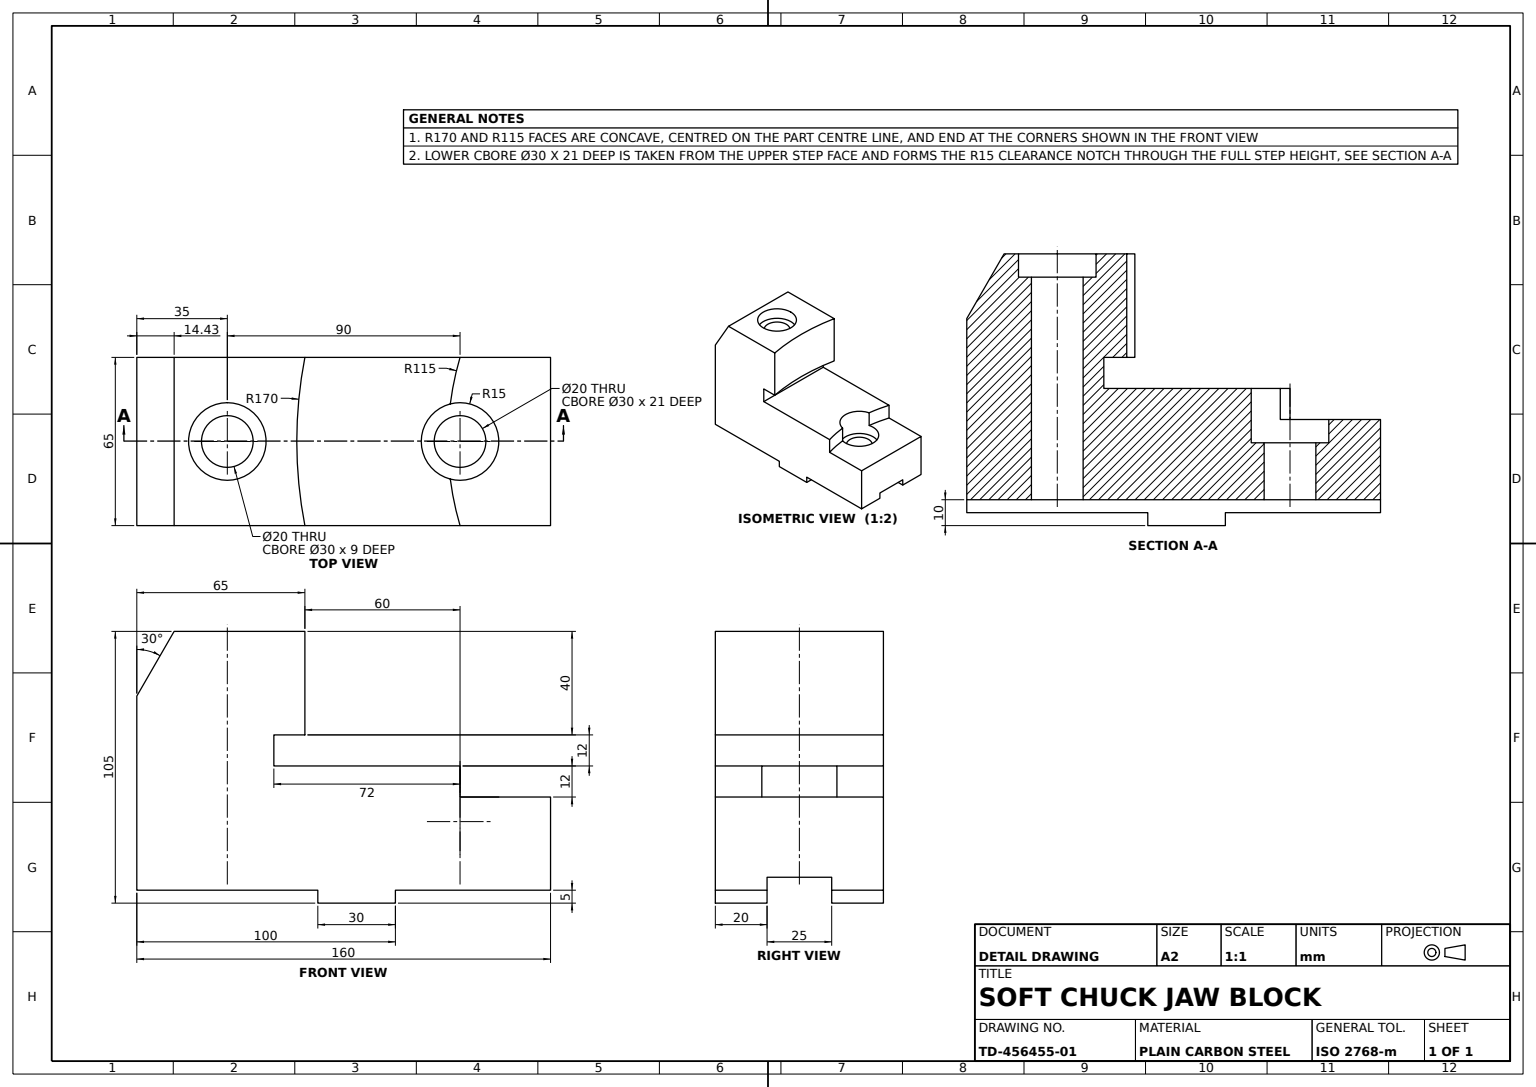
SolidWorks part; units mm, degrees
material "Plain Carbon Steel"
ref_plane "Front Plane" through (0, 0, 0) normal (0, 0, 1) x (1, 0, 0)
ref_plane "Top Plane" through (0, 0, 0) normal (0, 1, 0) x (1, 0, 0)
ref_plane "Right Plane" through (0, 0, 0) normal (1, 0, 0) x (0, 0, -1)
sketch "Stepped Profile Sketch" plane through (0, 0, 0) normal (0, 0, 1) x (1, 0, 0)
  line L0 (0, 0) -> (0, 75)
  line L1 (0, 75) -> (14.4338, 100)
  line L2 (14.4338, 100) -> (65, 100)
  line L3 (65, 100) -> (65, 60)
  line L4 (65, 48) -> (125, 48)
  line L5 (125, 48) -> (125, 36)
  line L6 (125, 36) -> (160, 36)
  line L7 (160, 36) -> (160, 0)
  line L8 (160, 0) -> (100, 0)
  line L9 (0, 75) -> (0, 132.9231) construction
  line L10 (65, 48) -> (53, 48)
  line L11 (53, 48) -> (53, 60)
  line L12 (53, 60) -> (65, 60)
  line L13 (70, 0) -> (70, -5)
  line L14 (70, -5) -> (100, -5)
  line L15 (100, -5) -> (100, 0)
  line L16 (70, 0) -> (0, 0)
  dimension "D1" = 100
  dimension "D2" = 30
  dimension "D3" = 25
  dimension "D4" = 65
  dimension "D5" = 12
  dimension "D6" = 40
  dimension "D7" = 160
  dimension "D8" = 35
  dimension "D9" = 12
  dimension "D10" = 12
  dimension "D11" = 30
  dimension "D12" = 60
  dimension "D13" = 5
extrude "Stepped Block Body" add sketch "Stepped Profile Sketch" along normal blind 65
sketch "Relief Cut Sketch" plane through (160, 0, 0) normal (1, 0, 0) x (0, 0, -1)
  line L0 (-65, 0) -> (0, 0) construction
  line L2 (-45, 0) -> (-45, 5)
  line L3 (-45, 5) -> (-20, 5)
  line L4 (-20, 0) -> (-20, 5)
  line L5 (-65, 0) -> (-65, 36) construction
  line L6 (0, 0) -> (0, 36) construction
  line L7 (-45, 0) -> (-45, -9.0383)
  line L8 (-45, -9.0383) -> (-20, -9.0383)
  line L9 (-20, -9.0383) -> (-20, 0)
  line L10 (-65, 36) -> (0, 36) construction
  dimension "D1" = 20
  dimension "D2" = 20
  dimension "D3" = 5
  dimension "D4" = 45.0383
extrude "Relief Cut 20x20" cut sketch "Relief Cut Sketch" against normal through all
sketch "Arc Cut 115 Sketch" plane through (0, 48, 0) normal (0, 1, 0) x (1, 0, 0)
  line L0 (160, -65) -> (160, 0) construction
  circle A0 centre (235.3121, -32.5) radius 115
  point P6 (160, -32.5)
  dimension "D1" = 115
extrude "Arc Cut 115" cut sketch "Arc Cut 115 Sketch" against normal up to surface (12 mm away) up to face at (142.5, 36, 32.5)
sketch "Arc Cut 170 Sketch" plane through (0, 100, 0) normal (0, 1, 0) x (1, 0, 0)
  line L0 (14.4338, -65) -> (14.4338, 0) construction
  circle A0 centre (231.8645, -32.5) radius 170
  point P5 (14.4338, -32.5)
  dimension "D1" = 170
extrude "Arc Cut 170" cut sketch "Arc Cut 170 Sketch" against normal up to surface (40 mm away) up to face at (59, 60, 32.5)
sketch "Upper Hole Location" plane through (0, 36, 0) normal (0, 1, 0) x (1, 0, 0)
  line L0 (160, -65) -> (160, 0) construction
  line L1 (160, -65) -> (125, -65) construction
  point P0 (125, -32.5)
  dimension "D1" = 35
  dimension "D2" = 32.5
hole_wizard "Upper C-Bore Hole Ø20" positions "3DSketch4" profile "Sketch11" legacy
sketch3d "3DSketch4"
  point P0 (125, 36, 32.5)
sketch "Sketch11" plane through (125, 36, 32.5) normal (1, 0, 0) x (0, 0, 1)
  line L0 (0, 0) -> (0, 99.8749)
  line L1 (0, 99.8749) -> (10, 99.8749)
  line L2 (10, 99.8749) -> (10, 9)
  line L3 (10, 9) -> (15, 9)
  line L4 (15, 9) -> (15, 0)
  line L5 (15, 0) -> (0, 0)
  line L6 (0, 110) -> (0, -10) construction
  dimension "Diameter" = 20
  dimension "Depth" = 100
  dimension "C-Bore Diameter" = 30
  dimension "C-Bore Depth" = 9
sketch "Lower Hole Location" plane through (0, 100, 0) normal (0, 1, 0) x (1, 0, 0)
  line L0 (14.4338, -65) -> (14.4338, 0) construction
  point P0 (35, -32.5)
  point P3 (14.4338, -32.5)
  dimension "D1" = 90
hole_wizard "Lower C-Bore Hole Ø20" positions "3DSketch5" profile "Sketch14" legacy
sketch3d "3DSketch5"
  point P0 (35, 100, 32.5)
sketch "Sketch14" plane through (35, 100, 32.5) normal (1, 0, 0) x (0, 0, 1)
  line L0 (0, 0) -> (0, 99.8749)
  line L1 (0, 99.8749) -> (10, 99.8749)
  line L2 (10, 99.8749) -> (10, 9)
  line L3 (10, 9) -> (15, 9)
  line L4 (15, 9) -> (15, 0)
  line L5 (15, 0) -> (0, 0)
  line L6 (0, 110) -> (0, -10) construction
  dimension "Diameter" = 20
  dimension "Depth" = 100
  dimension "C-Bore Diameter" = 30
  dimension "C-Bore Depth" = 9
sketch "Hole Clearance Notch Sketch" plane through (0, 48, 0) normal (0, 1, 0) x (1, 0, 0)
  circle A2 centre (125, -32.5) radius 15 construction
  circle A3 centre (125, -32.5) radius 15
extrude "Hole Clearance Notch" cut sketch "Hole Clearance Notch Sketch" against normal up to surface (12 mm away) up to face at (138.4188, 36, 32.5)
